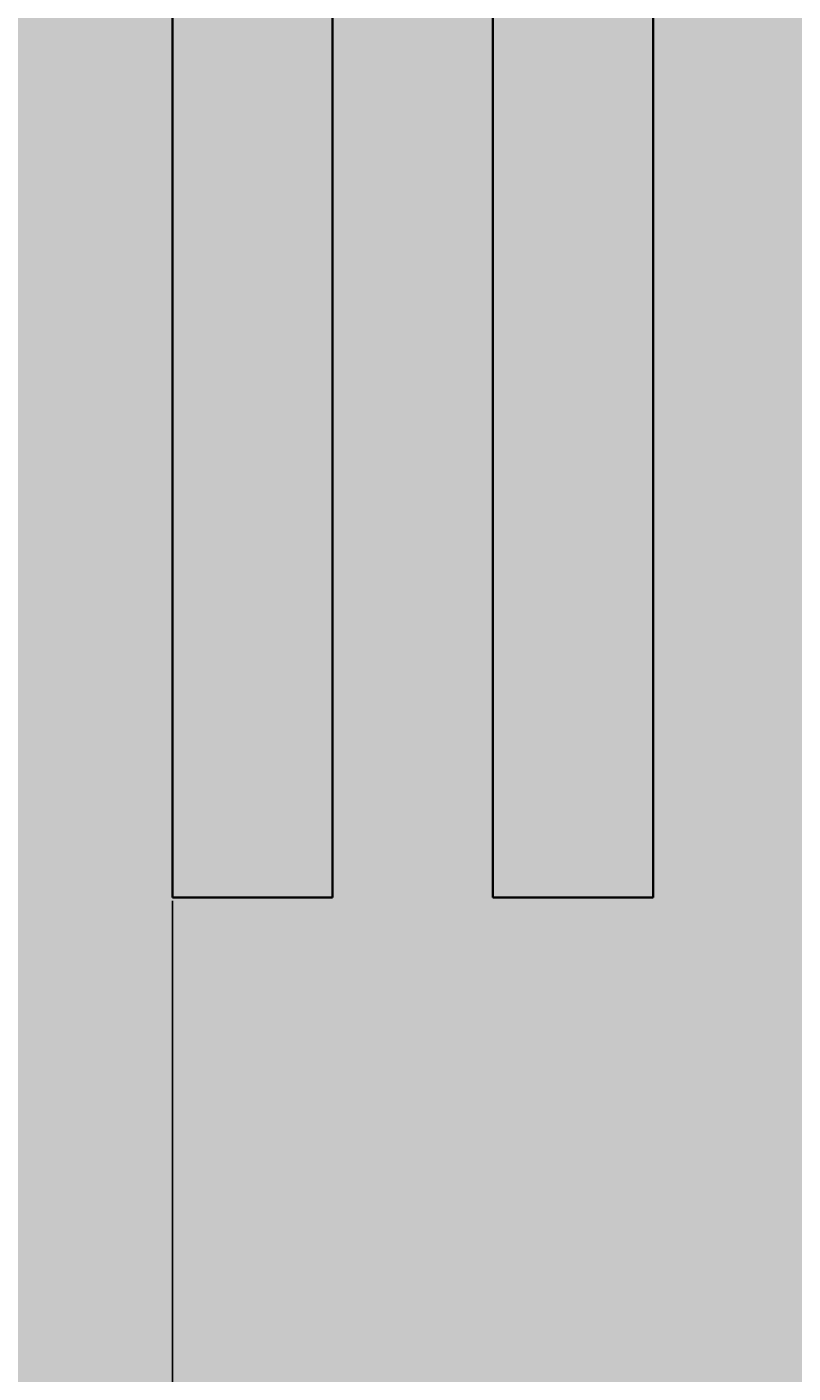
# Model space of a CAD drawing. Units: inches. Extents: x -1 to 292, y -3 to 199.
# Tile 19 of 52: x 68 to 82, y 42 to 68. Entities that reach past the tile are written whole.
import ezdxf

# ---------------------------------------------------------------- set-up
doc = ezdxf.new("R2010")
doc.units = ezdxf.units.IN
doc.header["$MEASUREMENT"] = 0
for name, color, linetype, lineweight in [('M-DIMS', 2, 'Continuous', 18), ('M-EQPM', 7, 'Continuous', 35), ('M-PATT', 8, 'Continuous', 13)]:
    doc.layers.add(name, color=color, linetype=linetype, lineweight=lineweight)
doc.styles.get("Standard").update_dxf_attribs({"font": 'arial.ttf'})
doc.dimstyles.get("Standard").update_dxf_attribs({"dimtxt": 0.18, "dimasz": 0.18, "dimexe": 0.18, "dimexo": 0.0625, "dimgap": 0.09, "dimtad": 0, "dimtih": 1, "dimtoh": 1, "dimdec": 4, "dimzin": 0, "dimdsep": 46, "dimtxsty": 'Standard', "dimcen": 0.09, "dimadec": 0, "dimazin": 0, "dimtfac": 1, "dimtdec": 4, "dimtofl": 0, "dimtmove": 0, "dimatfit": 3, "dimfxl": 1, "dimtolj": 1, "dimtzin": 0, "dimarcsym": 0})

# ---------------------------------------------------------------- blocks, each defined once
blk = doc.blocks.new('BOILER-TUBE')
for p, q in [((0, 40.63), (0, 0)), ((3, 40.63), (3, 0))]:
    blk.add_line(p, q)
blk.add_lwpolyline([(3, 0), (0, 0)])
blk = doc.blocks.new('*D7')
at = {"layer": 'Defpoints', "color": 0, "transparency": 16777216}
for p in [(21.861, 54.582), (205.115, 54.582), (21.861, 39.982)]:
    blk.add_point(p, dxfattribs=at)
at = {"layer": 'M-DIMS', "color": 0, "lineweight": -2, "transparency": 16777216}
for p, q in [((21.861, 54.52), (21.861, 39.802)), ((205.115, 54.52), (205.115, 39.802)), ((22.041, 39.982), (113.033, 39.982)), ((204.935, 39.982), (113.944, 39.982))]:
    blk.add_line(p, q, dxfattribs=at)
at = {"layer": 'M-DIMS', "color": 0, "transparency": 16777216}
for points in [[(22.041, 40.012), (22.041, 39.952), (21.861, 39.982)], [(204.935, 40.012), (204.935, 39.952), (205.115, 39.982)]]:
    blk.add_solid(points, dxfattribs=at)
at = {"layer": 'M-DIMS', "color": 0, "transparency": 16777216, "insert": (113.488, 39.982), "char_height": 0.18, "attachment_point": 5}
blk.add_mtext('\\A1;183.25', dxfattribs=at)
blk = doc.blocks.new('*D8')
at = {"layer": 'Defpoints', "color": 0, "transparency": 16777216}
for p in [(-0.662, 126.765), (111.488, 126.765), (69.013, 25.514)]:
    blk.add_point(p, dxfattribs=at)
at = {"layer": 'M-DIMS', "color": 0, "lineweight": -2, "transparency": 16777216}
for p, q in [((111.426, 126.765), (-0.842, 126.765)), ((-0.662, 126.585), (-0.662, 76.321)), ((-0.662, 25.694), (-0.662, 75.958)), ((68.951, 25.514), (-0.842, 25.514))]:
    blk.add_line(p, q, dxfattribs=at)
at = {"layer": 'M-DIMS', "color": 0, "transparency": 16777216}
for points in [[(-0.692, 126.585), (-0.632, 126.585), (-0.662, 126.765)], [(-0.692, 25.694), (-0.632, 25.694), (-0.662, 25.514)]]:
    blk.add_solid(points, dxfattribs=at)
at = {"layer": 'M-DIMS', "color": 0, "transparency": 16777216, "insert": (-0.662, 76.14), "char_height": 0.18, "attachment_point": 5}
blk.add_mtext('\\A1;101.25', dxfattribs=at)
blk = doc.blocks.new('*D20')
at = {"layer": 'Defpoints', "color": 0, "transparency": 16777216}
for p in [(64.679, 51.267), (70.679, 51.267), (70.679, -2.71)]:
    blk.add_point(p, dxfattribs=at)
at = {"layer": 'M-DIMS', "color": 0, "lineweight": -2, "transparency": 16777216}
for p, q in [((64.679, 51.205), (64.679, -2.89)), ((70.679, 51.205), (70.679, -2.89)), ((64.859, -2.71), (67.529, -2.71)), ((70.499, -2.71), (67.828, -2.71))]:
    blk.add_line(p, q, dxfattribs=at)
at = {"layer": 'M-DIMS', "color": 0, "transparency": 16777216}
for points in [[(64.859, -2.68), (64.859, -2.74), (64.679, -2.71)], [(70.499, -2.68), (70.499, -2.74), (70.679, -2.71)]]:
    blk.add_solid(points, dxfattribs=at)
at = {"layer": 'M-DIMS', "color": 0, "transparency": 16777216, "insert": (67.679, -2.71), "char_height": 0.18, "attachment_point": 5}
blk.add_mtext('\\A1;6', dxfattribs=at)

msp = doc.modelspace()

# ---------------------------------------------------------------- hatches: boundary and pattern name
at = {"layer": 'M-PATT'}
h = msp.add_hatch(color=256, dxfattribs=at)
h.set_gradient(color1=(237, 31, 36), color2=(242, 113, 114), tint=1, name='CYLINDER')
h.paths.add_polyline_path([(106.0735, 105.9941), (106.0735, 106.9941), (108.0603, 106.9941), (107.8488, 107.6501), (57.8007, 107.6501, 0.4142136), (49.9241, 99.7735), (52.3176, 101.3278), (55.0097, 99.7735), (57.4032, 101.3278), (60.0953, 99.7735), (62.4888, 101.3278), (65.1809, 99.7735), (67.5744, 101.3278), (70.2665, 99.7735), (72.66, 101.3278), (75.3521, 99.7735), (77.7456, 101.3278), (80.4377, 99.7735), (82.8312, 101.3278), (85.5233, 99.7735), (87.9168, 101.3278), (90.6089, 99.7735), (93.0024, 101.3278), (95.6945, 99.7735), (98.088, 101.3278), (100.7801, 99.7735), (103.1736, 101.3278), (105.8657, 99.7735), (108.2592, 101.3278), (110.9513, 99.7735), (113.3448, 101.3278), (116.0369, 99.7735), (118.4304, 101.3278), (121.1225, 99.7735), (123.516, 101.3278), (126.2082, 99.7735), (128.6016, 101.3278), (131.2938, 99.7735), (133.6872, 101.3278), (136.3794, 99.7735), (138.7728, 101.3278), (141.465, 99.7735), (143.8584, 101.3278), (146.5506, 99.7735), (148.944, 101.3278), (151.6362, 99.7735), (154.0296, 101.3278), (156.7218, 99.7735), (159.1152, 101.3278), (160.6222, 100.4578), (160.6222, 107.6501), (115.4883, 107.6501), (115.4883, 106.9941), (120.9032, 106.9941), (120.9032, 105.9941), (120.9032, 103.3981), (106.0735, 103.3981)])
h.paths.add_polyline_path([(169.176, 107.6501), (162.1623, 107.6501), (162.1623, 100.004), (164.2008, 101.3278), (166.893, 99.7735), (169.2864, 101.3278), (171.9786, 99.7735), (174.372, 101.3278), (177.0526, 99.7802, 0.4139642)])
h.paths.add_polyline_path([(111.4883, 107.6501), (107.8488, 107.6501), (108.0603, 106.9941), (111.4883, 106.9941)], flags=17)
h.paths.add_polyline_path([(61.6788, 91.897), (57.8007, 91.897, -0.1099266), (54.4604, 92.6403), (43.2011, 92.6403), (23.9502, 84.4688), (23.9502, 58.376), (43.2011, 47.2615), (50.9409, 47.2615, -0.2705926), (57.8007, 51.2672), (61.6788, 51.2672)])
h.paths.add_polyline_path([(73.6788, 91.897), (70.6788, 91.897), (70.6788, 51.2672), (73.6788, 51.2672)])
h.paths.add_polyline_path([(79.6788, 91.897), (76.6788, 91.897), (76.6788, 51.2672), (79.6788, 51.2672)])
h.paths.add_polyline_path([(67.6788, 91.897), (64.6788, 91.897), (64.6788, 51.2672), (67.6788, 51.2672)])
h.paths.add_polyline_path([(101.6788, 91.897), (82.6788, 91.897), (82.6788, 51.2672), (101.6788, 51.2672)])
h.paths.add_polyline_path([(107.6788, 91.897), (104.6788, 91.897), (104.6788, 51.2672), (107.6788, 51.2672)])
h.paths.add_polyline_path([(113.6788, 91.897), (110.6788, 91.897), (110.6788, 51.2672), (113.6788, 51.2672)])
h.paths.add_polyline_path([(119.6788, 91.897), (116.6788, 91.897), (116.6788, 51.2672), (119.6788, 51.2672)])
h.paths.add_polyline_path([(141.6788, 91.897), (122.6788, 91.897), (122.6788, 51.2672), (141.6788, 51.2672)])
h.paths.add_polyline_path([(147.6788, 91.897), (144.6788, 91.897), (144.6788, 51.2672), (147.6788, 51.2672)])
h.paths.add_polyline_path([(153.6788, 91.897), (150.6788, 91.897), (150.6788, 51.2672), (153.6788, 51.2672)])
h.paths.add_polyline_path([(159.6788, 91.897), (156.6788, 91.897), (156.6788, 51.2672), (159.6788, 51.2672)])
h.paths.add_polyline_path([(179.5897, 92.6403), (172.5163, 92.6403, -0.1099266), (169.176, 91.897), (162.6788, 91.897), (162.6788, 51.2672), (169.176, 51.2672, -0.2705926), (176.0358, 47.2615), (179.5897, 47.2615)])
h.paths.add_polyline_path([(203.0265, 84.4688), (183.7755, 92.6403), (181.5897, 92.6403), (181.5897, 47.2615), (183.7755, 47.2615), (203.0265, 58.376)])
h.paths.add_polyline_path([(184.4188, 61.52), (200.7224, 61.52), (200.7224, 77.7532), (184.4188, 77.7532)], flags=24)
h = msp.add_hatch(color=256, dxfattribs=at)
h.set_gradient(color1=(0, 255, 255), color2=(0, 255, 255), tint=1)
h.paths.add_polyline_path([(75.3521, 99.7735), (72.66, 101.3278), (70.2665, 99.7735), (67.5744, 101.3278), (65.1809, 99.7735), (62.4888, 101.3278), (60.0953, 99.7735), (57.4032, 101.3278), (55.0097, 99.7735), (52.3176, 101.3278), (49.9241, 99.7735, 0.4142136), (57.8007, 91.897), (61.6788, 91.897), (61.6788, 51.2672), (57.8007, 51.2672, 0.8088808), (54.5813, 36.2021), (65.0947, 51.2672), (64.6788, 51.2672), (64.6788, 91.897), (67.6788, 91.897), (67.6788, 51.2672), (65.0947, 51.2672), (54.5813, 36.2021, 0.1056561), (57.8007, 35.5141), (169.176, 35.5141, 1), (169.176, 51.2672), (162.6788, 51.2672), (162.6788, 91.897), (169.176, 91.897, 0.4144629), (177.0526, 99.7802), (174.372, 101.3278), (171.9786, 99.7735), (169.2864, 101.3278), (166.893, 99.7735), (164.2008, 101.3278), (162.1623, 100.004), (162.1623, 96.1027), (160.6222, 96.1027), (160.6222, 100.4578), (159.1152, 101.3278), (156.7218, 99.7735), (154.0296, 101.3278), (151.6362, 99.7735), (148.944, 101.3278), (146.5506, 99.7735), (143.8584, 101.3278), (141.465, 99.7735), (138.7728, 101.3278), (136.3794, 99.7735), (133.6872, 101.3278), (131.2938, 99.7735), (128.6016, 101.3278), (126.2082, 99.7735), (123.516, 101.3278), (121.1225, 99.7735), (118.4304, 101.3278), (116.0369, 99.7735), (113.3448, 101.3278), (110.9513, 99.7735), (108.2592, 101.3278), (105.8657, 99.7735), (103.1736, 101.3278), (100.7801, 99.7735), (98.088, 101.3278), (95.6945, 99.7735), (93.0024, 101.3278), (90.6089, 99.7735), (87.9168, 101.3278), (85.5233, 99.7735), (82.8312, 101.3278), (80.4377, 99.7735), (77.7456, 101.3278)])
h.paths.add_polyline_path([(79.6788, 91.897), (79.6788, 51.2672), (76.6788, 51.2672), (76.6788, 91.897)], flags=16)
h.paths.add_polyline_path([(73.6788, 91.897), (73.6788, 51.2672), (70.6788, 51.2672), (70.6788, 91.897)], flags=16)
h.paths.add_polyline_path([(82.6788, 91.897), (101.6788, 91.897), (101.6788, 51.2672), (82.6788, 51.2672)], flags=16)
h.paths.add_polyline_path([(104.6788, 91.897), (107.6788, 91.897), (107.6788, 51.2672), (104.6788, 51.2672)], flags=16)
h.paths.add_polyline_path([(110.6788, 91.897), (113.6788, 91.897), (113.6788, 51.2672), (110.6788, 51.2672)], flags=16)
h.paths.add_polyline_path([(116.6788, 91.897), (119.6788, 91.897), (119.6788, 51.2672), (116.6788, 51.2672)], flags=16)
h.paths.add_polyline_path([(122.6788, 91.897), (141.6788, 91.897), (141.6788, 51.2672), (144.6788, 51.2672), (144.6788, 91.897), (147.6788, 91.897), (147.6788, 51.2672), (122.6788, 51.2672)], flags=16)
h.paths.add_polyline_path([(150.6788, 91.897), (153.6788, 91.897), (153.6788, 51.2672), (150.6788, 51.2672)], flags=16)
h.paths.add_polyline_path([(156.6788, 91.897), (159.6788, 91.897), (159.6788, 51.2672), (156.6788, 51.2672)], flags=16)

# ---------------------------------------------------------------- block references
at = {"layer": 'M-EQPM'}
for p in [(70.679, 51.267), (76.679, 51.267)]:
    msp.add_blockref('BOILER-TUBE', p, dxfattribs=at)

# ---------------------------------------------------------------- dimensions: what is measured, and where the dimension line sits
at = {"layer": 'M-DIMS'}
for base, p1, p2, angle, picture, middle in [((-0.6625, 126.765), (69.013, 25.5141), (111.4883, 126.765), 90, '*D8', (-0.6625, 76.1396)), ((21.8612, 39.9821), (205.1155, 54.5821), (21.8612, 54.5821), 180, '*D7', (113.4883, 39.9821))]:
    dim = msp.add_linear_dim(base=base, p1=p1, p2=p2, angle=angle, dimstyle='Standard', override={"dimdec": 2, "dimlfac": 1, "dimrnd": 0, "dimzin": 0, "dimdsep": 46, "dimlunit": 2}, dxfattribs=at)
    dim.commit()
    dim.dimension.update_dxf_attribs({"geometry": picture, "text_midpoint": middle})
dim = msp.add_linear_dim(base=(70.6788, -2.7104), p1=(64.6788, 51.2672), p2=(70.6788, 51.2672), dimstyle='Standard', override={"dimdec": 0, "dimlfac": 1, "dimrnd": 0, "dimzin": 0, "dimdsep": 46, "dimlunit": 2}, dxfattribs=at)
dim.commit()
dim.dimension.update_dxf_attribs({"geometry": '*D20', "text_midpoint": (67.6788, -2.7104)})

doc.saveas('drawing.dxf')
